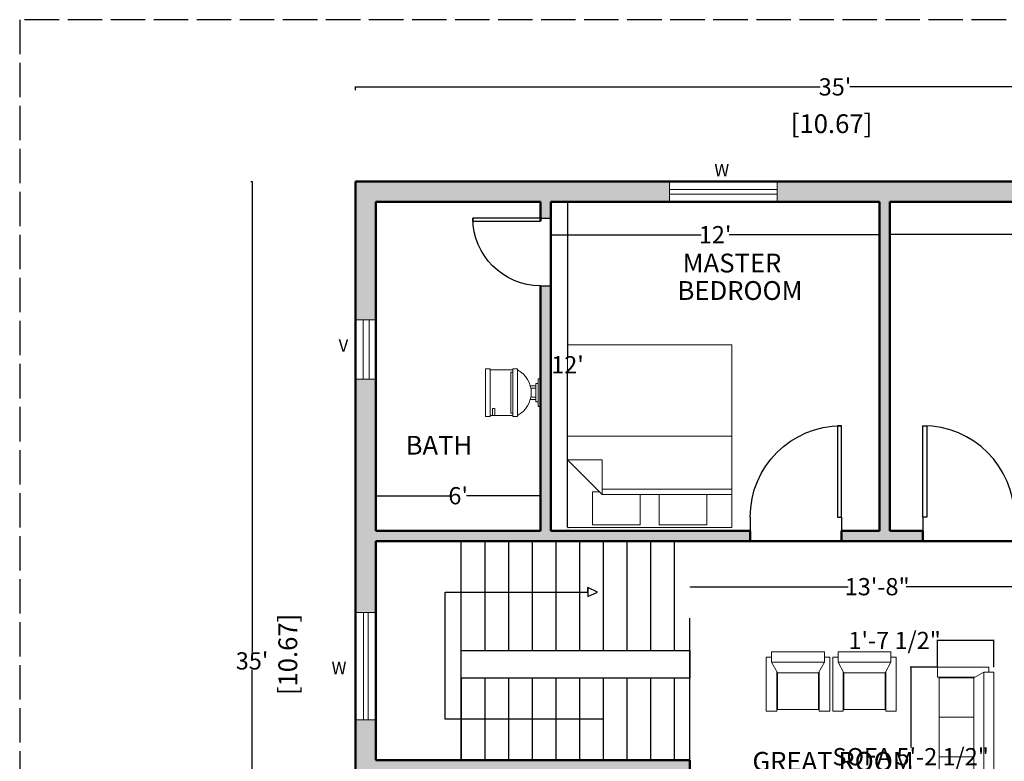
# Model space of a CAD drawing. Units: inches. Extents: x 2905 to 3459, y 4225 to 4672.
# Tile 2 of 3: x 2905 to 3248, y 4414 to 4672. Entities that reach past the tile are written whole.
import ezdxf

# ---------------------------------------------------------------- set-up
doc = ezdxf.new("R2010")
doc.units = ezdxf.units.IN
doc.header["$MEASUREMENT"] = 0
doc.linetypes.add('ACAD_ISO02W100', pattern=[15, 12, -3])
doc.layers.get('0').update_dxf_attribs({"color": 252})
for name, color, linetype, lineweight in [('A-ANNO-DIMS', 2, 'Continuous', 18), ('A-ANNO-TEXT', 7, 'Continuous', 18), ('A-ANNO-TTLB', 7, 'ACAD_ISO02W100', 25), ('A-AREA-IDEN', 7, 'Continuous', 25), ('A-DOOR', 3, 'Continuous', 25), ('A-FLOR-FIXT', 9, 'Continuous', 18), ('A-FLOR-STRS', 7, 'Continuous', 25), ('A-GLAZ', 4, 'Continuous', 18), ('A-WALL-PATT', 251, 'Continuous', 13), ('furniture', 8, 'Continuous', 18), ('walls', 251, 'Continuous', 50)]:
    doc.layers.add(name, color=color, linetype=linetype, lineweight=lineweight)
doc.styles.get("Standard").update_dxf_attribs({"font": 'arial.ttf'})
doc.dimstyles.get("Standard").update_dxf_attribs({"dimtxt": 6, "dimasz": 0.18, "dimexe": 0.18, "dimexo": 0.0625, "dimgap": 0.09, "dimtad": 0, "dimtih": 1, "dimtoh": 1, "dimzin": 0, "dimdsep": 46, "dimlunit": 3, "dimtxsty": 'Standard', "dimcen": 0.09, "dimadec": 0, "dimazin": 0, "dimtfac": 1, "dimtofl": 0, "dimtmove": 0, "dimatfit": 3, "dimfxl": 1, "dimtolj": 1, "dimtzin": 0, "dimarcsym": 0})

# ---------------------------------------------------------------- blocks, each defined once
blk = doc.blocks.new('*U2')
for p, q in [((0, 0), (0, -6)), ((40, 0), (40, -6))]:
    blk.add_line(p, q)
blk.add_lwpolyline([(0, 0), (0, 40), (1.75, 40), (1.75, 0)], close=True)
blk.add_arc((0, 0), 40, 0, 90)
blk = doc.blocks.new('BEDK')
at = {"layer": 'furniture'}
for p, q in [((315470.08, -113271.37), (315550.08, -113271.37)), ((315470.08, -113271.37), (315470.08, -113343.37)), ((315499.68, -113271.37), (315484.48, -113286.57)), ((315499.68, -113286.57), (315499.68, -113271.37)), ((315510.08, -113343.37), (315510.08, -113271.37)), ((315550.08, -113271.37), (315550.08, -113343.37)), ((315471.28, -113303.17), (315471.28, -113282.37)), ((315471.28, -113282.37), (315485.68, -113282.37)), ((315485.68, -113282.37), (315485.68, -113285.37)), ((315484.48, -113286.57), (315499.68, -113286.57)), ((315484.48, -113343.37), (315484.48, -113286.57)), ((315486.88, -113286.57), (315486.88, -113343.37)), ((315484.48, -113303.17), (315471.28, -113303.17)), ((315471.28, -113332.37), (315471.28, -113311.57)), ((315471.28, -113311.57), (315484.48, -113311.57)), ((315484.48, -113332.37), (315471.28, -113332.37)), ((315550.08, -113343.37), (315470.08, -113343.37))]:
    blk.add_line(p, q, dxfattribs=at)
blk = doc.blocks.new('*U4')
for p, q in [((-10, 22), (-10, 12)), ((10, 12), (10, 22)), ((-10, 21), (-7, 21)), ((-7, 20), (-10, 20)), ((-7, 21), (-7, 20)), ((9, 13), (-9, 13)), ((-9, 13), (-9, 12)), ((9, 12), (9, 13)), ((10.5, 12), (-10.5, 12)), ((-10.5, 10), (-10.5, 12)), ((10.5, 10), (-10.5, 10)), ((10.5, 12), (10.5, 10)), ((-3, 4.4065), (-3, 2)), ((3, 2), (3, 4.4065)), ((4, 2), (-4, 2)), ((-4, 2), (-4, 1)), ((-2, 2), (-2, 4.1658)), ((2, 4.1658), (2, 2)), ((4, 1), (4, 2))]:
    blk.add_line(p, q)
for points in [[(10.5, 22), (10.5, 24), (-10.5, 24), (-10.5, 22)], [(6, 0), (6, 1), (-6, 1), (-6, 0)]]:
    blk.add_lwpolyline(points, close=True)
blk.add_arc((0, 15.3333), 11.3333, 208.0725, 331.9275)
blk = doc.blocks.new('FABRIC SOFA 1S')
at = {"layer": 'furniture'}
for p, q in [((3, 18.12), (34, 18.12)), ((3, 15.12), (3, 18.12)), ((34, 12.12), (34, 18.12)), ((0, -15.12), (0, 15.12)), ((6, 15.12), (0, 15.12)), ((6, -15.12), (6, 15.12)), ((12, 11.75), (6, 15.12)), ((11.33, 12.12), (34, 12.12)), ((6, -15.12), (0, -15.12)), ((3, -18.12), (3, -15.12)), ((6, -15.12), (12, -11.75)), ((11.33, -12.12), (34, -12.12)), ((34, -12.12), (34, -18.12)), ((3, -18.12), (34, -18.12))]:
    blk.add_line(p, q, dxfattribs=at)
blk.add_lwpolyline([(12, -11.75), (12, 11.75), (33, 11.75), (33, -11.75)], close=True, dxfattribs=at)
blk = doc.blocks.new('FABRIC SOFA 4S')
at = {"layer": 'furniture'}
for p, q in [((3, 54), (34, 54)), ((3, 51), (3, 54)), ((34, 48), (34, 54)), ((0, -51), (0, 51)), ((6, 51), (0, 51)), ((6, -51), (6, 51)), ((12, 47.63), (6, 51)), ((11.14, 48), (34, 48)), ((33, 23.81), (12, 23.81)), ((33, 0), (12, 0)), ((33, -23.81), (12, -23.81)), ((6, -51), (0, -51)), ((3, -54), (3, -51)), ((6, -51), (12, -47.63)), ((11.54, -48), (34, -48)), ((34, -48), (34, -54)), ((3, -54), (34, -54))]:
    blk.add_line(p, q, dxfattribs=at)
blk.add_lwpolyline([(12, -47.63), (12, 47.63), (33, 47.63), (33, -47.63)], close=True, dxfattribs=at)
blk = doc.blocks.new('*D11')
at = {"layer": 'A-ANNO-DIMS', "color": 0, "lineweight": -2, "transparency": 16777216}
for p, q in [((3028.98, 4506.51), (3028.98, 4506.62)), ((3029.16, 4506.44), (3054.77, 4506.44)), ((3086.11, 4506.44), (3060.5, 4506.44)), ((3086.29, 4506.51), (3086.29, 4506.62))]:
    blk.add_line(p, q, dxfattribs=at)
at = {"layer": 'A-ANNO-DIMS', "color": 0, "transparency": 16777216}
for points in [[(3029.16, 4506.47), (3029.16, 4506.41), (3028.98, 4506.44)], [(3086.11, 4506.47), (3086.11, 4506.41), (3086.29, 4506.44)]]:
    blk.add_solid(points, dxfattribs=at)
at = {"layer": 'Defpoints', "color": 0, "transparency": 16777216}
for p in [(3028.98, 4506.44), (3086.29, 4506.44), (3086.29, 4506.44)]:
    blk.add_point(p, dxfattribs=at)
at = {"layer": 'A-ANNO-DIMS', "color": 0, "transparency": 16777216, "insert": (3057.63, 4506.44), "char_height": 6, "attachment_point": 5}
blk.add_mtext("\\A1;6'", dxfattribs=at)
blk = doc.blocks.new('*D12')
at = {"layer": 'A-ANNO-DIMS', "color": 0, "lineweight": -2, "transparency": 16777216}
for p, q in [((3089.87, 4597.49), (3089.87, 4597.61)), ((3090.05, 4597.43), (3142.27, 4597.43)), ((3204.29, 4597.43), (3152.07, 4597.43)), ((3204.47, 4597.49), (3204.47, 4597.61))]:
    blk.add_line(p, q, dxfattribs=at)
at = {"layer": 'A-ANNO-DIMS', "color": 0, "transparency": 16777216}
for points in [[(3090.05, 4597.46), (3090.05, 4597.4), (3089.87, 4597.43)], [(3204.29, 4597.46), (3204.29, 4597.4), (3204.47, 4597.43)]]:
    blk.add_solid(points, dxfattribs=at)
at = {"layer": 'Defpoints', "color": 0, "transparency": 16777216}
for p in [(3089.87, 4597.43), (3204.47, 4597.43), (3204.47, 4597.43)]:
    blk.add_point(p, dxfattribs=at)
at = {"layer": 'A-ANNO-DIMS', "color": 0, "transparency": 16777216, "insert": (3147.17, 4597.43), "char_height": 6, "attachment_point": 5}
blk.add_mtext("\\A1;12'", dxfattribs=at)
blk = doc.blocks.new('*D13')
at = {"layer": 'A-ANNO-DIMS', "color": 0, "lineweight": -2, "transparency": 16777216}
for p, q in [((3097.24, 4608.83), (3095.55, 4608.83)), ((3095.73, 4608.65), (3095.73, 4555.2)), ((3095.73, 4495.54), (3095.73, 4548.99)), ((3095.79, 4495.36), (3095.91, 4495.36))]:
    blk.add_line(p, q, dxfattribs=at)
at = {"layer": 'A-ANNO-DIMS', "color": 0, "transparency": 16777216}
for points in [[(3095.7, 4608.65), (3095.76, 4608.65), (3095.73, 4608.83)], [(3095.7, 4495.54), (3095.76, 4495.54), (3095.73, 4495.36)]]:
    blk.add_solid(points, dxfattribs=at)
at = {"layer": 'Defpoints', "color": 0, "transparency": 16777216}
for p in [(3097.31, 4608.83), (3095.73, 4495.36), (3095.73, 4495.36)]:
    blk.add_point(p, dxfattribs=at)
at = {"layer": 'A-ANNO-DIMS', "color": 0, "transparency": 16777216, "insert": (3095.73, 4552.09), "char_height": 6, "attachment_point": 5}
blk.add_mtext("\\A1;12'", dxfattribs=at)
blk = doc.blocks.new('*D14')
at = {"layer": 'A-ANNO-DIMS', "color": 0, "lineweight": -2, "transparency": 16777216}
for p, q in [((3208.05, 4597.69), (3208.05, 4597.8)), ((3208.23, 4597.62), (3268.37, 4597.62)), ((3348.73, 4597.62), (3288.59, 4597.62)), ((3348.91, 4597.69), (3348.91, 4597.8))]:
    blk.add_line(p, q, dxfattribs=at)
at = {"layer": 'A-ANNO-DIMS', "color": 0, "transparency": 16777216}
for points in [[(3208.23, 4597.65), (3208.23, 4597.59), (3208.05, 4597.62)], [(3348.73, 4597.65), (3348.73, 4597.59), (3348.91, 4597.62)]]:
    blk.add_solid(points, dxfattribs=at)
at = {"layer": 'Defpoints', "color": 0, "transparency": 16777216}
for p in [(3208.05, 4597.62), (3348.91, 4597.62), (3348.91, 4597.62)]:
    blk.add_point(p, dxfattribs=at)
at = {"layer": 'A-ANNO-DIMS', "color": 0, "transparency": 16777216, "insert": (3278.48, 4597.62), "char_height": 6, "attachment_point": 5}
blk.add_mtext('\\A1;14\'-6"', dxfattribs=at)
blk = doc.blocks.new('*D23')
at = {"layer": 'A-ANNO-DIMS', "color": 0, "lineweight": -2, "transparency": 16777216}
for p, q in [((3138.38, 4474.67), (3138.38, 4474.55)), ((3138.56, 4474.73), (3193.54, 4474.73)), ((3268.75, 4474.73), (3213.77, 4474.73)), ((3268.93, 4474.79), (3268.93, 4474.91))]:
    blk.add_line(p, q, dxfattribs=at)
at = {"layer": 'A-ANNO-DIMS', "color": 0, "transparency": 16777216}
for points in [[(3138.56, 4474.76), (3138.56, 4474.7), (3138.38, 4474.73)], [(3268.75, 4474.76), (3268.75, 4474.7), (3268.93, 4474.73)]]:
    blk.add_solid(points, dxfattribs=at)
at = {"layer": 'Defpoints', "color": 0, "transparency": 16777216}
for p in [(3138.38, 4474.73), (3268.93, 4474.73), (3268.93, 4474.73)]:
    blk.add_point(p, dxfattribs=at)
at = {"layer": 'A-ANNO-DIMS', "color": 0, "transparency": 16777216, "insert": (3203.66, 4474.73), "char_height": 6, "attachment_point": 5}
blk.add_mtext('\\A1;13\'-8"', dxfattribs=at)
blk = doc.blocks.new('*D25')
at = {"layer": 'A-ANNO-DIMS', "color": 0, "lineweight": -2, "transparency": 16777216}
for p, q in [((2985.39, 4615.99), (2985.98, 4615.99)), ((2985.8, 4615.81), (2985.8, 4452.02)), ((2985.8, 4281.92), (2985.8, 4445.71)), ((2985.39, 4281.74), (2985.98, 4281.74))]:
    blk.add_line(p, q, dxfattribs=at)
at = {"layer": 'A-ANNO-DIMS', "color": 0, "transparency": 16777216}
for points in [[(2985.77, 4615.81), (2985.83, 4615.81), (2985.8, 4615.99)], [(2985.77, 4281.92), (2985.83, 4281.92), (2985.8, 4281.74)]]:
    blk.add_solid(points, dxfattribs=at)
at = {"layer": 'Defpoints', "color": 0, "transparency": 16777216}
for p in [(2985.32, 4615.99), (2985.32, 4281.74), (2985.8, 4281.74)]:
    blk.add_point(p, dxfattribs=at)
at = {"layer": 'A-ANNO-DIMS', "color": 0, "transparency": 16777216, "insert": (2985.8, 4448.86), "char_height": 6, "attachment_point": 5}
blk.add_mtext("\\A1;35'", dxfattribs=at)
blk = doc.blocks.new('*D26')
at = {"layer": 'A-ANNO-DIMS', "color": 0, "lineweight": -2, "transparency": 16777216}
for p, q in [((3021.82, 4647.77), (3021.82, 4649.13)), ((3022, 4648.95), (3183.77, 4648.95)), ((3355.89, 4648.95), (3194.13, 4648.95)), ((3356.07, 4647.77), (3356.07, 4649.13))]:
    blk.add_line(p, q, dxfattribs=at)
at = {"layer": 'A-ANNO-DIMS', "color": 0, "transparency": 16777216}
for points in [[(3022, 4648.98), (3022, 4648.92), (3021.82, 4648.95)], [(3355.89, 4648.98), (3355.89, 4648.92), (3356.07, 4648.95)]]:
    blk.add_solid(points, dxfattribs=at)
at = {"layer": 'Defpoints', "color": 0, "transparency": 16777216}
for p in [(3021.82, 4647.71), (3356.07, 4648.95), (3356.07, 4647.71)]:
    blk.add_point(p, dxfattribs=at)
at = {"layer": 'A-ANNO-DIMS', "color": 0, "transparency": 16777216, "insert": (3188.95, 4648.95), "char_height": 6, "attachment_point": 5}
blk.add_mtext("\\A1;35'", dxfattribs=at)
blk = doc.blocks.new('WIN-PLAN-STANDARD')
for p, q in [((0, 7.16), (0, 0)), ((37.45, 7.16), (0, 7.16)), ((0, 7.16), (0, 4.38)), ((37.45, 0), (37.45, 7.16)), ((0, 4.38), (37.45, 4.38)), ((37.45, 4.38), (37.45, 2.7)), ((0, 2.7), (37.45, 2.7)), ((0, 0), (37.45, 0))]:
    blk.add_line(p, q)
blk = doc.blocks.new('*D44')
at = {"layer": 'A-ANNO-DIMS', "color": 0, "lineweight": -2, "transparency": 16777216}
for p, q in [((3224.63, 4446.63), (3215.16, 4446.63)), ((3215.34, 4446.45), (3215.34, 4418.67)), ((3215.34, 4384.49), (3215.34, 4412.28)), ((3224.63, 4384.31), (3215.16, 4384.31))]:
    blk.add_line(p, q, dxfattribs=at)
at = {"layer": 'A-ANNO-DIMS', "color": 0, "transparency": 16777216}
for points in [[(3215.31, 4446.45), (3215.37, 4446.45), (3215.34, 4446.63)], [(3215.31, 4384.49), (3215.37, 4384.49), (3215.34, 4384.31)]]:
    blk.add_solid(points, dxfattribs=at)
at = {"layer": 'Defpoints', "color": 0, "transparency": 16777216}
for p in [(3224.69, 4446.63), (3215.34, 4384.31), (3224.69, 4384.31)]:
    blk.add_point(p, dxfattribs=at)
at = {"layer": 'A-ANNO-DIMS', "color": 0, "transparency": 16777216, "insert": (3215.34, 4415.47), "char_height": 6, "attachment_point": 5}
blk.add_mtext('\\A1;SOFA 5\'-2 1/2"', dxfattribs=at)
blk = doc.blocks.new('*D45')
at = {"layer": 'A-ANNO-DIMS', "color": 0, "lineweight": -2, "transparency": 16777216}
for p, q in [((3224.69, 4455.98), (3224.51, 4455.98)), ((3224.69, 4446.69), (3224.69, 4456.16)), ((3244.13, 4455.98), (3224.87, 4455.98)), ((3244.31, 4446.69), (3244.31, 4456.16))]:
    blk.add_line(p, q, dxfattribs=at)
at = {"layer": 'A-ANNO-DIMS', "color": 0, "transparency": 16777216}
for points in [[(3224.87, 4456.01), (3224.87, 4455.95), (3224.69, 4455.98)], [(3244.13, 4456.01), (3244.13, 4455.95), (3244.31, 4455.98)]]:
    blk.add_solid(points, dxfattribs=at)
at = {"layer": 'Defpoints', "color": 0, "transparency": 16777216}
for p in [(3224.69, 4455.98), (3224.69, 4446.63), (3244.31, 4446.63)]:
    blk.add_point(p, dxfattribs=at)
at = {"layer": 'A-ANNO-DIMS', "color": 0, "transparency": 16777216, "insert": (3209.74, 4455.98), "char_height": 6, "attachment_point": 5}
blk.add_mtext('\\A1;1\'-7 1/2"', dxfattribs=at)

msp = doc.modelspace()

# ---------------------------------------------------------------- hatches: boundary and pattern name
at = {"layer": 'A-WALL-PATT'}
h = msp.add_hatch(color=256, dxfattribs=at)
h.dxf.hatch_style = 1
h.paths.add_polyline_path([(3291.611, 4382.367), (3288.03, 4382.367), (3288.03, 4349.781), (3348.911, 4349.781), (3348.911, 4353.362), (3291.611, 4353.362)])
h.paths.add_polyline_path([(3291.611, 4410.662), (3288.03, 4410.662), (3288.03, 4405.956), (3291.611, 4405.956)])
h.paths.add_polyline_path([(3356.074, 4439.171), (3348.911, 4439.171), (3348.911, 4387.379), (3356.074, 4387.379)])
h.paths.add_polyline_path([(3356.074, 4366.687), (3348.911, 4366.687), (3348.911, 4288.899), (3341.991, 4288.899), (3341.991, 4286.512), (3341.991, 4281.737), (3356.074, 4281.737)])
h.paths.add_polyline_path([(3310.157, 4286.512, -0.0187698), (3310.247, 4288.899), (3286.75, 4288.899), (3286.75, 4281.737), (3310.157, 4281.737)])
h.paths.add_polyline_path([(3249.298, 4288.899), (3230.73, 4288.899), (3230.73, 4346.199), (3227.148, 4346.199), (3227.148, 4288.899), (3221.363, 4288.899), (3221.363, 4281.737), (3249.298, 4281.737)])
h.paths.add_polyline_path([(3230.73, 4349.781), (3227.148, 4349.781), (3227.148, 4346.199), (3230.73, 4346.199)])
h.paths.add_polyline_path([(3183.911, 4288.899), (3169.848, 4288.899), (3169.848, 4346.199), (3166.267, 4346.199), (3166.267, 4288.899), (3158.463, 4288.899), (3158.463, 4281.737), (3183.911, 4281.737)])
h.paths.add_polyline_path([(3169.848, 4349.781), (3166.267, 4349.781), (3166.267, 4346.199), (3169.848, 4346.199)])
h.paths.add_polyline_path([(3166.267, 4349.781), (3154.383, 4349.781), (3154.383, 4346.199), (3166.267, 4346.199)])
h.paths.add_polyline_path([(3130.507, 4349.781), (3105.385, 4349.781), (3105.385, 4288.899), (3082.76, 4288.899), (3082.76, 4281.737), (3121.011, 4281.737), (3121.011, 4288.899), (3108.967, 4288.899), (3108.967, 4346.199), (3130.507, 4346.199)])
h.paths.add_polyline_path([(3045.307, 4288.899), (3028.985, 4288.899), (3028.985, 4351.673), (3021.822, 4351.673), (3021.822, 4281.737), (3045.307, 4281.737)])
h.paths.add_polyline_path([(3028.985, 4428.302), (3021.822, 4428.302), (3021.822, 4389.126), (3028.985, 4389.126), (3028.985, 4410.662), (3138.383, 4410.662), (3138.383, 4414.244), (3028.985, 4414.244)])
h.paths.add_polyline_path([(3356.074, 4615.988), (3308.212, 4615.988), (3308.212, 4608.826), (3348.911, 4608.826), (3348.911, 4459.863), (3356.074, 4459.863)])
h.paths.add_polyline_path([(3053.98, 4501.489), (3061.351, 4501.489), (3061.351, 4511.329), (3053.98, 4511.329)], flags=9)
h.paths.add_polyline_path([(3141.419, 4592.43), (3152.5, 4592.43), (3152.5, 4602.27), (3141.419, 4602.27)], flags=9)
h.paths.add_polyline_path([(3089.982, 4547.099), (3101.063, 4547.099), (3101.063, 4556.939), (3089.982, 4556.939)], flags=9)
h.paths.add_polyline_path([(3268.583, 4592.669), (3287.963, 4592.669), (3287.963, 4602.509), (3268.583, 4602.509)], flags=9)
h.paths.add_polyline_path([(3307.047, 4423.398), (3314.418, 4423.398), (3314.418, 4433.237), (3307.047, 4433.237)], flags=9)
h.paths.add_polyline_path([(3288.865, 4462.697), (3316.591, 4462.697), (3316.591, 4472.539), (3288.865, 4472.539)], flags=9)
h.paths.add_polyline_path([(3037.676, 4519.097), (3065.402, 4519.097), (3065.402, 4528.939), (3037.676, 4528.939)], flags=9)
h.paths.add_polyline_path([(3265.13, 4583.219), (3291.666, 4583.219), (3291.666, 4593.397), (3265.13, 4593.397)], flags=9)
h.paths.add_polyline_path([(3257.487, 4572.872), (3308.243, 4572.872), (3308.243, 4583.057), (3257.487, 4583.057)], flags=9)
h.paths.add_polyline_path([(3132.382, 4572.872), (3183.138, 4572.872), (3183.138, 4583.057), (3132.382, 4583.057)], flags=9)
h.paths.add_polyline_path([(3134.197, 4582.452), (3175.785, 4582.452), (3175.785, 4592.629), (3134.197, 4592.629)], flags=9)
h = msp.add_hatch(color=256, dxfattribs=at)
h.dxf.hatch_style = 1
h.paths.add_polyline_path([(3208.048, 4608.826), (3270.759, 4608.826), (3270.759, 4615.988), (3168.781, 4615.988), (3168.781, 4608.826), (3204.467, 4608.826), (3204.467, 4494.225), (3191.238, 4494.225), (3191.238, 4490.644), (3219.587, 4490.644), (3219.587, 4494.225), (3208.048, 4494.225)])
h.paths.add_polyline_path([(3089.866, 4579.625), (3086.285, 4579.625), (3086.285, 4494.225), (3028.985, 4494.225), (3028.985, 4547.094), (3021.822, 4547.094), (3021.822, 4465.755), (3028.985, 4465.755), (3028.985, 4490.644), (3159.404, 4490.644), (3159.404, 4494.225), (3089.866, 4494.225)])
h.paths.add_polyline_path([(3131.329, 4615.988), (3021.822, 4615.988), (3021.822, 4567.786), (3024.467, 4567.786), (3028.985, 4567.786), (3028.985, 4608.826), (3086.285, 4608.826), (3086.285, 4603.214), (3086.328, 4603.214), (3089.866, 4603.214), (3089.866, 4608.826), (3131.329, 4608.826)])

# ---------------------------------------------------------------- linework, layer by layer
at = {"layer": 'A-ANNO-TTLB'}
for p, q in [((2904.821, 4672.373), (2904.821, 4225.241)), ((3458.552, 4672.373), (2904.821, 4672.373))]:
    msp.add_line(p, q, dxfattribs=at)
at = {"layer": 'A-FLOR-STRS'}
for p, q in [((3058.726, 4414.244), (3058.726, 4490.644)), ((3066.987, 4452.444), (3066.987, 4490.644)), ((3075.247, 4452.444), (3075.247, 4490.644)), ((3083.507, 4452.444), (3083.507, 4490.644)), ((3091.767, 4452.444), (3091.767, 4490.644)), ((3100.028, 4452.444), (3100.028, 4490.644)), ((3108.288, 4452.444), (3108.288, 4490.644)), ((3116.548, 4452.444), (3116.548, 4490.644)), ((3116.548, 4452.444), (3116.548, 4490.644)), ((3124.808, 4452.444), (3124.808, 4490.644)), ((3133.068, 4452.444), (3133.068, 4490.644)), ((3053.147, 4428.569), (3053.147, 4472.812)), ((3053.147, 4472.812), (3102.829, 4472.812)), ((3102.829, 4472.812), (3102.829, 4474.395)), ((3102.829, 4474.395), (3102.829, 4471.332)), ((3106.15, 4472.863), (3102.829, 4474.395)), ((3102.829, 4471.332), (3106.15, 4472.863)), ((3138.383, 4442.894), (3138.383, 4463.75)), ((3058.726, 4452.444), (3138.383, 4452.444)), ((3138.383, 4452.444), (3138.383, 4442.894)), ((3138.383, 4442.894), (3058.726, 4442.894)), ((3058.726, 4442.894), (3058.726, 4414.244)), ((3066.987, 4414.244), (3066.987, 4442.894)), ((3075.247, 4414.244), (3075.247, 4442.894)), ((3083.507, 4414.244), (3083.507, 4442.894)), ((3091.767, 4414.244), (3091.767, 4442.894)), ((3100.028, 4414.244), (3100.028, 4442.894)), ((3108.288, 4414.244), (3108.288, 4442.894)), ((3116.548, 4414.244), (3116.548, 4442.894)), ((3116.548, 4414.244), (3116.548, 4442.894)), ((3124.808, 4414.244), (3124.808, 4442.894)), ((3133.068, 4414.244), (3133.068, 4442.894)), ((3138.383, 4414.244), (3138.383, 4442.894)), ((3108.288, 4428.569), (3053.147, 4428.569))]:
    msp.add_line(p, q, dxfattribs=at)
at = {"layer": 'A-GLAZ'}
for p, q in [((3021.822, 4567.786), (3028.985, 4567.786)), ((3021.822, 4547.094), (3021.822, 4567.786)), ((3021.822, 4567.786), (3024.467, 4567.786)), ((3024.467, 4567.786), (3024.467, 4547.094)), ((3026.594, 4547.094), (3026.594, 4567.786)), ((3028.985, 4567.786), (3028.985, 4547.094)), ((3028.985, 4547.094), (3021.822, 4547.094)), ((3024.467, 4547.094), (3026.594, 4547.094))]:
    msp.add_line(p, q, dxfattribs=at)
at = {"layer": 'walls'}
for p, q in [((3021.822, 4615.988), (3356.074, 4615.988)), ((3021.822, 4281.737), (3021.822, 4615.988)), ((3028.985, 4608.826), (3086.285, 4608.826)), ((3028.985, 4494.225), (3028.985, 4608.826)), ((3086.285, 4602.182), (3086.285, 4608.826)), ((3089.866, 4494.225), (3089.866, 4608.826)), ((3089.866, 4608.826), (3204.467, 4608.826)), ((3204.467, 4494.225), (3204.467, 4608.826)), ((3208.048, 4494.225), (3208.048, 4608.826)), ((3208.048, 4608.826), (3348.911, 4608.826)), ((3086.285, 4494.225), (3086.285, 4579.625)), ((3028.985, 4494.225), (3086.285, 4494.225)), ((3089.866, 4494.225), (3159.404, 4494.225)), ((3159.404, 4494.225), (3159.404, 4490.644)), ((3191.238, 4494.225), (3204.467, 4494.225)), ((3191.238, 4494.225), (3191.238, 4490.644)), ((3208.048, 4494.225), (3219.587, 4494.225)), ((3219.587, 4494.225), (3219.587, 4490.644)), ((3028.985, 4490.644), (3268.93, 4490.644)), ((3028.985, 4414.244), (3028.985, 4490.644)), ((3028.985, 4414.244), (3138.383, 4414.244)), ((3138.383, 4414.244), (3138.383, 4410.662))]:
    msp.add_line(p, q, dxfattribs=at)

# ---------------------------------------------------------------- block references
at = {"layer": 'A-DOOR', "xscale": -0.58972064018156, "yscale": 0.58972064018156, "zscale": 0.58972064018156, "rotation": 90}
msp.add_blockref('*U2', (3086.328, 4603.214), dxfattribs=at)
at = {"layer": 'A-DOOR', "yscale": 0.7958373047019981, "zscale": 0.7958373047019981}
for p, xscale in [((3191.238, 4499), -0.7958373047019981), ((3219.587, 4499), 0.7958373047019981)]:
    msp.add_blockref('*U2', p, dxfattribs=dict(at, xscale=xscale))
at = {"layer": 'A-FLOR-FIXT', "xscale": 0.7958373047019981, "yscale": 0.7958373047019981, "zscale": 0.7958373047019981, "rotation": 90}
msp.add_blockref('*U4', (3086.285, 4542.365), dxfattribs=at)
at = {"layer": 'A-GLAZ'}
msp.add_blockref('WIN-PLAN-STANDARD', (3131.329, 4608.826), dxfattribs=at)
at = {"layer": 'A-GLAZ', "rotation": 89.99999999999491}
msp.add_blockref('WIN-PLAN-STANDARD', (3028.984, 4428.302), dxfattribs=at)
at = {"layer": 'furniture'}
for name, p, xscale, yscale, zscale, rotation in [('BEDK', (-87049.852, -246567.499), 0.7958373047019981, 0.7958373047019981, 0.7958373047019981, 89.99999999999996), ('FABRIC SOFA 1S', (3176.067, 4452.038), 0.6103067503488249, 0.6103067503488249, 0.6103067503488249, 270), ('FABRIC SOFA 1S', (3199.23, 4452.038), 0.6103067503488249, 0.6103067503488249, 0.6103067503488249, 270), ('FABRIC SOFA 4S', (3244.312, 4415.471), 0.5770400048926188, 0.5770400048926188, 0.5770400048926188, 180)]:
    msp.add_blockref(name, p, dxfattribs=dict(at, xscale=xscale, yscale=yscale, zscale=zscale, rotation=rotation))

# ---------------------------------------------------------------- texts
at = {"layer": 'A-ANNO-DIMS'}
msp.add_text('[10.67]', height=6.5613, dxfattribs=at).set_placement((3173.542, 4632.837))
msp.add_text('[10.67]', height=6.5613, rotation=90, dxfattribs=at).set_placement((3001.541, 4436.896))
at = {"layer": 'A-ANNO-TEXT'}
for s, p in [('W', (3146.902, 4617.796)), ('V', (3015.949, 4556.661)), ('W', (3013.514, 4444.217))]:
    msp.add_text(s, height=4.319, dxfattribs=at).set_placement(p)
at = {"layer": 'A-AREA-IDEN'}
for s, p in [('MASTER', (3135.893, 4584.26)), ('BEDROOM', (3134.079, 4574.682)), ('BATH', (3039.316, 4520.738)), ('GREAT ROOM', (3160.193, 4410.561))]:
    msp.add_text(s, height=6.5613, dxfattribs=at).set_placement(p)

# ---------------------------------------------------------------- dimensions: what is measured, and where the dimension line sits
at = {"layer": 'A-ANNO-DIMS'}
for base, p1, p2, text, picture, middle in [((3356.074, 4648.949), (3021.822, 4647.711), (3356.074, 4647.711), "35'", '*D26', (3188.948, 4648.949)), ((3348.911, 4597.623), (3208.048, 4597.623), (3348.911, 4597.623), '14\'-6"', '*D14', (3278.48, 4597.623)), ((3204.467, 4597.425), (3089.866, 4597.425), (3204.467, 4597.425), "12'", '*D12', (3147.167, 4597.425)), ((3086.285, 4506.443), (3028.985, 4506.443), (3086.285, 4506.443), "6'", '*D11', (3057.635, 4506.443)), ((3268.93, 4474.73), (3138.383, 4474.73), (3268.93, 4474.73), '13\'-8"', '*D23', (3203.657, 4474.73))]:
    dim = msp.add_linear_dim(base=base, p1=p1, p2=p2, text=text, dimstyle='Standard', override={"dimclrd": 0, "dimclre": 0, "dimclrt": 0}, dxfattribs=at)
    dim.commit()
    dim.dimension.update_dxf_attribs({"geometry": picture, "text_midpoint": middle})
for base, p1, p2, angle, text, override, picture, middle in [((2985.804, 4281.737), (2985.324, 4615.988), (2985.324, 4281.737), 90, "35'", {"dimclrd": 0, "dimclre": 0, "dimclrt": 0}, '*D25', (2985.804, 4448.862)), ((3095.729, 4495.362), (3097.307, 4608.826), (3095.729, 4495.362), 90, "12'", {"dimclrd": 0, "dimclre": 0, "dimclrt": 0}, '*D13', (3095.729, 4552.094)), ((3215.345, 4384.311), (3224.693, 4446.631), (3224.693, 4384.311), 270, 'SOFA <>', {"dimdec": 1, "dimlfac": 1, "dimrnd": 0, "dimzin": 1, "dimdsep": 46, "dimlunit": 4, "dimfrac": 2}, '*D44', (3215.345, 4415.471))]:
    dim = msp.add_linear_dim(base=base, p1=p1, p2=p2, angle=angle, text=text, dimstyle='Standard', override=override, dxfattribs=at)
    dim.commit()
    dim.dimension.update_dxf_attribs({"geometry": picture, "text_midpoint": middle})
dim = msp.add_linear_dim(base=(3224.693, 4455.979), p1=(3244.312, 4446.631), p2=(3224.693, 4446.631), angle=180, dimstyle='Standard', override={"dimdec": 1, "dimlfac": 1, "dimrnd": 0, "dimzin": 1, "dimdsep": 46, "dimlunit": 4, "dimfrac": 2}, dxfattribs=at)
dim.commit()
dim.dimension.update_dxf_attribs({"geometry": '*D45', "text_midpoint": (3209.74, 4455.979)})

doc.saveas('drawing.dxf')
